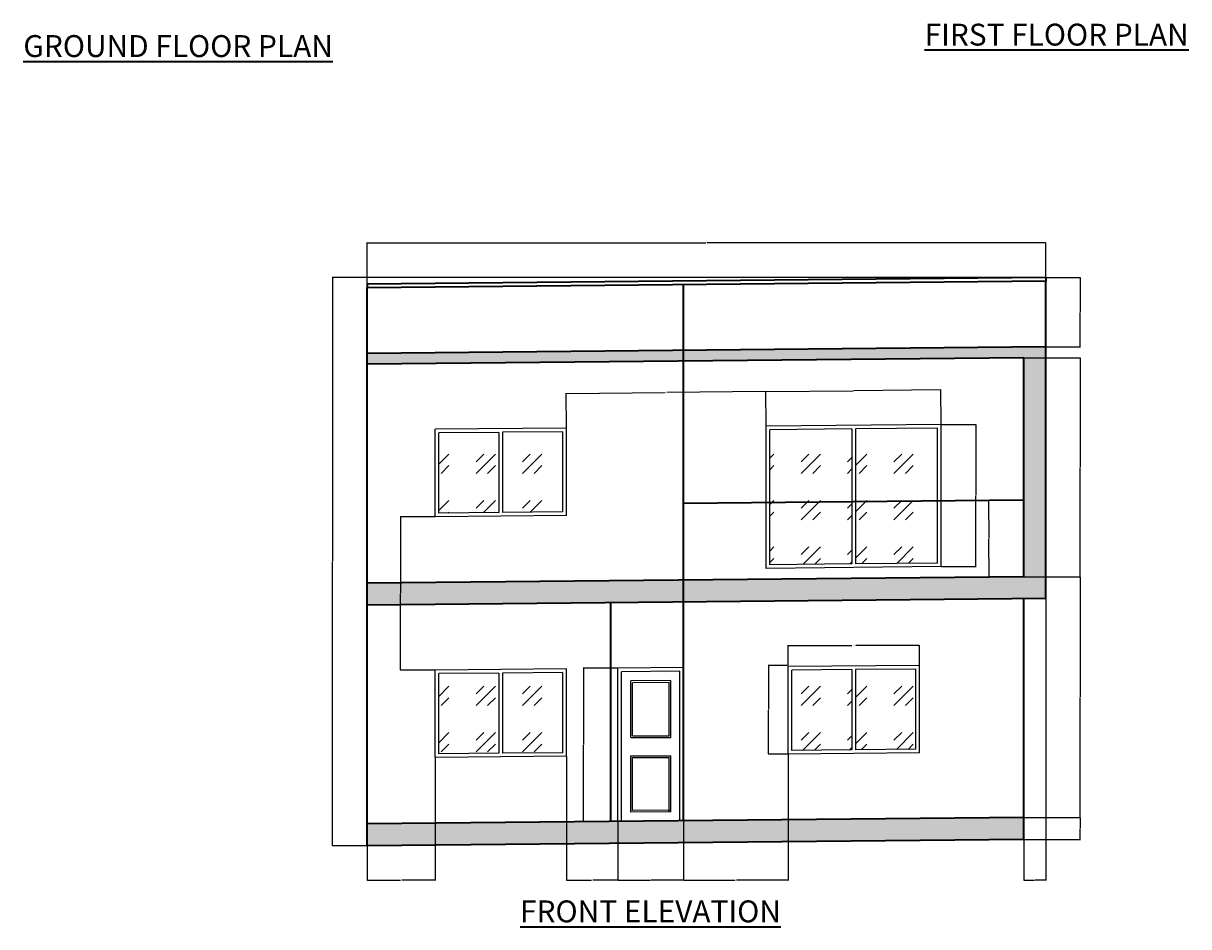
# Model space of a CAD drawing. Units: inches. Extents: x 2831 to 3729, y 3926 to 4974.
# Tile 1 of 8: x 2934 to 3573, y 3926 to 4422. Entities that reach past the tile are written whole.
import ezdxf

# ---------------------------------------------------------------- set-up
doc = ezdxf.new("R2010")
doc.units = ezdxf.units.IN
for name, color, linetype, lineweight in [('A-ANNO-DIMS', 2, 'Continuous', 18), ('A-ANNO-TEXT', 7, 'Continuous', 35), ('A-DOOR', 3, 'Continuous', 25), ('A-ELEV', 7, 'Continuous', 35), ('A-ELEV-PATT', 252, 'Continuous', 13), ('A-GLAZ', 4, 'Continuous', 25), ('A-GLAZ-PATT', 9, 'Continuous', 13)]:
    doc.layers.add(name, color=color, linetype=linetype, lineweight=lineweight)
doc.styles.get("Standard").update_dxf_attribs({"font": 'arial.ttf'})
doc.dimstyles.get("Standard").update_dxf_attribs({"dimtxt": 0.18, "dimasz": 0.18, "dimexe": 0.18, "dimexo": 0.0625, "dimgap": 0.09, "dimtad": 0, "dimtih": 1, "dimtoh": 1, "dimdec": 4, "dimzin": 0, "dimdsep": 46, "dimtxsty": 'Standard', "dimcen": 0.09, "dimadec": 0, "dimazin": 0, "dimtfac": 1, "dimtdec": 4, "dimtofl": 0, "dimtmove": 0, "dimatfit": 3, "dimfxl": 1, "dimtolj": 1, "dimtzin": 0, "dimarcsym": 0})

# ---------------------------------------------------------------- blocks, each defined once
blk = doc.blocks.new('WINDOW-72X48IN-ELEV')
for p, q in [((0, 48), (72, 48.7)), ((0, 48), (0, 0)), ((2, 46.02), (35, 46.34)), ((2, 46.02), (2, 2.02)), ((35, 2.34), (35, 46.34)), ((37, 46.36), (70, 46.68)), ((37, 2.36), (37, 46.36)), ((70, 46.68), (70, 2.68)), ((72, 48.7), (72, 0.7)), ((0, 0), (72, 0.7)), ((2, 2.02), (35, 2.34)), ((37, 2.36), (70, 2.68))]:
    blk.add_line(p, q)
blk = doc.blocks.new('*D27')
at = {"layer": 'A-ANNO-DIMS', "color": 0, "lineweight": -2, "transparency": 16777216}
for p, q in [((3353.06, 4069.58), (3353.06, 4080.49)), ((3353.24, 4080.31), (3387.94, 4080.31)), ((3424.88, 4080.31), (3390.18, 4080.31)), ((3425.06, 4069.58), (3425.06, 4080.49))]:
    blk.add_line(p, q, dxfattribs=at)
at = {"layer": 'A-ANNO-DIMS', "color": 0, "transparency": 16777216}
for points in [[(3353.24, 4080.34), (3353.24, 4080.28), (3353.06, 4080.31)], [(3424.88, 4080.34), (3424.88, 4080.28), (3425.06, 4080.31)]]:
    blk.add_solid(points, dxfattribs=at)
at = {"layer": 'Defpoints', "color": 0, "transparency": 16777216}
for p in [(3353.06, 4080.31), (3353.06, 4069.51), (3425.06, 4069.51)]:
    blk.add_point(p, dxfattribs=at)
at = {"layer": 'A-ANNO-DIMS', "color": 0, "transparency": 16777216, "insert": (3389.06, 4080.31), "char_height": 0.18, "attachment_point": 5}
blk.add_mtext('\\A1;WINDOW 72 TYP.', dxfattribs=at)
blk = doc.blocks.new('*D28')
at = {"layer": 'A-ANNO-DIMS', "color": 0, "lineweight": -2, "transparency": 16777216}
for p, q in [((3352.99, 4069.51), (3342.08, 4069.51)), ((3342.26, 4069.33), (3342.26, 4045.34)), ((3342.26, 4020.99), (3342.26, 4044.98)), ((3352.99, 4020.81), (3342.08, 4020.81))]:
    blk.add_line(p, q, dxfattribs=at)
at = {"layer": 'A-ANNO-DIMS', "color": 0, "transparency": 16777216}
for points in [[(3342.23, 4069.33), (3342.29, 4069.33), (3342.26, 4069.51)], [(3342.23, 4020.99), (3342.29, 4020.99), (3342.26, 4020.81)]]:
    blk.add_solid(points, dxfattribs=at)
at = {"layer": 'Defpoints', "color": 0, "transparency": 16777216}
for p in [(3353.06, 4069.51), (3342.26, 4020.81), (3353.06, 4020.81)]:
    blk.add_point(p, dxfattribs=at)
at = {"layer": 'A-ANNO-DIMS', "color": 0, "transparency": 16777216, "insert": (3342.26, 4045.16), "char_height": 0.18, "attachment_point": 5}
blk.add_mtext('\\A1;49 TYP.', dxfattribs=at)
blk = doc.blocks.new('*D62')
at = {"layer": 'A-ANNO-DIMS', "color": 0, "lineweight": -2, "transparency": 16777216}
for p, q in [((3122.29, 4278.64), (3122.29, 4301.33)), ((3122.47, 4301.15), (3308, 4301.15)), ((3494.11, 4301.15), (3308.58, 4301.15)), ((3494.29, 4282.26), (3494.29, 4301.33))]:
    blk.add_line(p, q, dxfattribs=at)
at = {"layer": 'A-ANNO-DIMS', "color": 0, "transparency": 16777216}
for points in [[(3122.47, 4301.18), (3122.47, 4301.12), (3122.29, 4301.15)], [(3494.11, 4301.18), (3494.11, 4301.12), (3494.29, 4301.15)]]:
    blk.add_solid(points, dxfattribs=at)
at = {"layer": 'Defpoints', "color": 0, "transparency": 16777216}
for p in [(3494.29, 4301.15), (3494.29, 4282.2), (3122.29, 4278.58)]:
    blk.add_point(p, dxfattribs=at)
at = {"layer": 'A-ANNO-DIMS', "color": 0, "transparency": 16777216, "insert": (3308.29, 4301.15), "char_height": 0.18, "attachment_point": 5}
blk.add_mtext('\\A1;372', dxfattribs=at)
blk = doc.blocks.new('*D63')
at = {"layer": 'A-ANNO-DIMS', "color": 0, "lineweight": -2, "transparency": 16777216}
for p, q in [((3494.23, 4282.2), (3103.16, 4282.2)), ((3103.34, 4282.02), (3103.34, 4126.56)), ((3103.34, 3970.75), (3103.34, 4126.2)), ((3122.24, 3970.57), (3103.16, 3970.57))]:
    blk.add_line(p, q, dxfattribs=at)
at = {"layer": 'A-ANNO-DIMS', "color": 0, "transparency": 16777216}
for points in [[(3103.31, 4282.02), (3103.37, 4282.02), (3103.34, 4282.2)], [(3103.31, 3970.75), (3103.37, 3970.75), (3103.34, 3970.57)]]:
    blk.add_solid(points, dxfattribs=at)
at = {"layer": 'Defpoints', "color": 0, "transparency": 16777216}
for p in [(3103.34, 4282.2), (3494.29, 4282.2), (3122.31, 3970.57)]:
    blk.add_point(p, dxfattribs=at)
at = {"layer": 'A-ANNO-DIMS', "color": 0, "transparency": 16777216, "insert": (3103.34, 4126.38), "char_height": 0.18, "attachment_point": 5}
blk.add_mtext('\\A1;311.6', dxfattribs=at)
blk = doc.blocks.new('*D64')
at = {"layer": 'A-ANNO-DIMS', "color": 0, "lineweight": -2, "transparency": 16777216}
for p, q in [((3482.37, 3986.07), (3513.44, 3986.07)), ((3513.26, 3985.89), (3513.26, 3980.25)), ((3482.37, 3974.07), (3513.44, 3974.07)), ((3513.26, 3974.25), (3513.26, 3979.89))]:
    blk.add_line(p, q, dxfattribs=at)
at = {"layer": 'A-ANNO-DIMS', "color": 0, "transparency": 16777216}
for points in [[(3513.23, 3985.89), (3513.29, 3985.89), (3513.26, 3986.07)], [(3513.23, 3974.25), (3513.29, 3974.25), (3513.26, 3974.07)]]:
    blk.add_solid(points, dxfattribs=at)
at = {"layer": 'Defpoints', "color": 0, "transparency": 16777216}
for p in [(3482.31, 3986.07), (3513.26, 3986.07), (3482.31, 3974.07)]:
    blk.add_point(p, dxfattribs=at)
at = {"layer": 'A-ANNO-DIMS', "color": 0, "transparency": 16777216, "insert": (3513.26, 3980.07), "char_height": 0.18, "attachment_point": 5}
blk.add_mtext('\\A1;12', dxfattribs=at)
blk = doc.blocks.new('*D65')
at = {"layer": 'A-ANNO-DIMS', "color": 0, "lineweight": -2, "transparency": 16777216}
for p, q in [((3482.37, 4118.07), (3513.44, 4118.07)), ((3513.26, 4117.89), (3513.26, 4052.25)), ((3513.26, 3986.25), (3513.26, 4051.89)), ((3482.37, 3986.07), (3513.44, 3986.07))]:
    blk.add_line(p, q, dxfattribs=at)
at = {"layer": 'A-ANNO-DIMS', "color": 0, "transparency": 16777216}
for points in [[(3513.23, 4117.89), (3513.29, 4117.89), (3513.26, 4118.07)], [(3513.23, 3986.25), (3513.29, 3986.25), (3513.26, 3986.07)]]:
    blk.add_solid(points, dxfattribs=at)
at = {"layer": 'Defpoints', "color": 0, "transparency": 16777216}
for p in [(3482.31, 4118.07), (3513.26, 4118.07), (3482.31, 3986.07)]:
    blk.add_point(p, dxfattribs=at)
at = {"layer": 'A-ANNO-DIMS', "color": 0, "transparency": 16777216, "insert": (3513.26, 4052.07), "char_height": 0.18, "attachment_point": 5}
blk.add_mtext('\\A1;132', dxfattribs=at)
blk = doc.blocks.new('*D66')
at = {"layer": 'A-ANNO-DIMS', "color": 0, "lineweight": -2, "transparency": 16777216}
for p, q in [((3482.37, 4238.08), (3513.44, 4238.08)), ((3513.26, 4237.9), (3513.26, 4178.26)), ((3513.26, 4118.25), (3513.26, 4177.89)), ((3482.37, 4118.07), (3513.44, 4118.07))]:
    blk.add_line(p, q, dxfattribs=at)
at = {"layer": 'A-ANNO-DIMS', "color": 0, "transparency": 16777216}
for points in [[(3513.23, 4237.9), (3513.29, 4237.9), (3513.26, 4238.08)], [(3513.23, 4118.25), (3513.29, 4118.25), (3513.26, 4118.07)]]:
    blk.add_solid(points, dxfattribs=at)
at = {"layer": 'Defpoints', "color": 0, "transparency": 16777216}
for p in [(3482.31, 4238.08), (3513.26, 4238.08), (3482.31, 4118.07)]:
    blk.add_point(p, dxfattribs=at)
at = {"layer": 'A-ANNO-DIMS', "color": 0, "transparency": 16777216, "insert": (3513.26, 4178.08), "char_height": 0.18, "attachment_point": 5}
blk.add_mtext('\\A1;120', dxfattribs=at)
blk = doc.blocks.new('*D67')
at = {"layer": 'A-ANNO-DIMS', "color": 0, "lineweight": -2, "transparency": 16777216}
for p, q in [((3494.35, 4282.2), (3513.44, 4282.2)), ((3513.26, 4282.02), (3513.26, 4263.38)), ((3513.26, 4244.38), (3513.26, 4263.01)), ((3494.37, 4244.2), (3513.44, 4244.2))]:
    blk.add_line(p, q, dxfattribs=at)
at = {"layer": 'A-ANNO-DIMS', "color": 0, "transparency": 16777216}
for points in [[(3513.23, 4282.02), (3513.29, 4282.02), (3513.26, 4282.2)], [(3513.23, 4244.38), (3513.29, 4244.38), (3513.26, 4244.2)]]:
    blk.add_solid(points, dxfattribs=at)
at = {"layer": 'Defpoints', "color": 0, "transparency": 16777216}
for p in [(3494.29, 4282.2), (3513.26, 4282.2), (3494.31, 4244.2)]:
    blk.add_point(p, dxfattribs=at)
at = {"layer": 'A-ANNO-DIMS', "color": 0, "transparency": 16777216, "insert": (3513.26, 4263.2), "char_height": 0.18, "attachment_point": 5}
blk.add_mtext('\\A1;38', dxfattribs=at)
blk = doc.blocks.new('*D68')
at = {"layer": 'A-ANNO-DIMS', "color": 0, "lineweight": -2, "transparency": 16777216}
for p, q in [((3159.56, 4018.87), (3159.56, 3951.44)), ((3122.31, 3970.5), (3122.31, 3951.44)), ((3122.49, 3951.62), (3140.54, 3951.62)), ((3159.38, 3951.62), (3141.33, 3951.62))]:
    blk.add_line(p, q, dxfattribs=at)
at = {"layer": 'A-ANNO-DIMS', "color": 0, "transparency": 16777216}
for points in [[(3122.49, 3951.65), (3122.49, 3951.59), (3122.31, 3951.62)], [(3159.38, 3951.65), (3159.38, 3951.59), (3159.56, 3951.62)]]:
    blk.add_solid(points, dxfattribs=at)
at = {"layer": 'Defpoints', "color": 0, "transparency": 16777216}
for p in [(3159.56, 4018.93), (3122.31, 3970.57), (3159.56, 3951.62)]:
    blk.add_point(p, dxfattribs=at)
at = {"layer": 'A-ANNO-DIMS', "color": 0, "transparency": 16777216, "insert": (3140.93, 3951.62), "char_height": 0.18, "attachment_point": 5}
blk.add_mtext('\\A1;37.25', dxfattribs=at)
blk = doc.blocks.new('*D69')
at = {"layer": 'A-ANNO-DIMS', "color": 0, "lineweight": -2, "transparency": 16777216}
for p, q in [((3231.56, 4019.57), (3231.56, 3951.44)), ((3259.81, 3983.84), (3259.81, 3951.44)), ((3231.74, 3951.62), (3245.29, 3951.62)), ((3259.63, 3951.62), (3246.08, 3951.62))]:
    blk.add_line(p, q, dxfattribs=at)
at = {"layer": 'A-ANNO-DIMS', "color": 0, "transparency": 16777216}
for points in [[(3231.74, 3951.65), (3231.74, 3951.59), (3231.56, 3951.62)], [(3259.63, 3951.65), (3259.63, 3951.59), (3259.81, 3951.62)]]:
    blk.add_solid(points, dxfattribs=at)
at = {"layer": 'Defpoints', "color": 0, "transparency": 16777216}
for p in [(3231.56, 4019.63), (3259.81, 3983.9), (3259.81, 3951.62)]:
    blk.add_point(p, dxfattribs=at)
at = {"layer": 'A-ANNO-DIMS', "color": 0, "transparency": 16777216, "insert": (3245.68, 3951.62), "char_height": 0.18, "attachment_point": 5}
blk.add_mtext('\\A1;28.25', dxfattribs=at)
blk = doc.blocks.new('*D70')
at = {"layer": 'A-ANNO-DIMS', "color": 0, "lineweight": -2, "transparency": 16777216}
for p, q in [((3259.81, 3983.84), (3259.81, 3951.44)), ((3295.81, 3984.19), (3295.81, 3951.44)), ((3259.99, 3951.62), (3277.59, 3951.62)), ((3295.63, 3951.62), (3278.03, 3951.62))]:
    blk.add_line(p, q, dxfattribs=at)
at = {"layer": 'A-ANNO-DIMS', "color": 0, "transparency": 16777216}
for points in [[(3259.99, 3951.65), (3259.99, 3951.59), (3259.81, 3951.62)], [(3295.63, 3951.65), (3295.63, 3951.59), (3295.81, 3951.62)]]:
    blk.add_solid(points, dxfattribs=at)
at = {"layer": 'Defpoints', "color": 0, "transparency": 16777216}
for p in [(3259.81, 3983.9), (3295.81, 3984.25), (3295.81, 3951.62)]:
    blk.add_point(p, dxfattribs=at)
at = {"layer": 'A-ANNO-DIMS', "color": 0, "transparency": 16777216, "insert": (3277.81, 3951.62), "char_height": 0.18, "attachment_point": 5}
blk.add_mtext('\\A1;36', dxfattribs=at)
blk = doc.blocks.new('*D71')
at = {"layer": 'A-ANNO-DIMS', "color": 0, "lineweight": -2, "transparency": 16777216}
for p, q in [((3353.06, 4020.75), (3353.06, 3951.44)), ((3295.81, 3984.19), (3295.81, 3951.44)), ((3295.99, 3951.62), (3324.04, 3951.62)), ((3352.88, 3951.62), (3324.83, 3951.62))]:
    blk.add_line(p, q, dxfattribs=at)
at = {"layer": 'A-ANNO-DIMS', "color": 0, "transparency": 16777216}
for points in [[(3295.99, 3951.65), (3295.99, 3951.59), (3295.81, 3951.62)], [(3352.88, 3951.65), (3352.88, 3951.59), (3353.06, 3951.62)]]:
    blk.add_solid(points, dxfattribs=at)
at = {"layer": 'Defpoints', "color": 0, "transparency": 16777216}
for p in [(3353.06, 4020.81), (3295.81, 3984.25), (3353.06, 3951.62)]:
    blk.add_point(p, dxfattribs=at)
at = {"layer": 'A-ANNO-DIMS', "color": 0, "transparency": 16777216, "insert": (3324.43, 3951.62), "char_height": 0.18, "attachment_point": 5}
blk.add_mtext('\\A1;57.25', dxfattribs=at)
blk = doc.blocks.new('*D72')
at = {"layer": 'A-ANNO-DIMS', "color": 0, "lineweight": -2, "transparency": 16777216}
for p, q in [((3341.06, 4200.77), (3340.87, 4219.83)), ((3341.05, 4219.65), (3388.65, 4220.12)), ((3436.69, 4220.58), (3389.09, 4220.12)), ((3437.06, 4201.7), (3436.87, 4220.77))]:
    blk.add_line(p, q, dxfattribs=at)
at = {"layer": 'A-ANNO-DIMS', "color": 0, "transparency": 16777216}
for points in [[(3341.05, 4219.68), (3341.05, 4219.62), (3340.87, 4219.65)], [(3436.69, 4220.61), (3436.69, 4220.55), (3436.87, 4220.59)]]:
    blk.add_solid(points, dxfattribs=at)
at = {"layer": 'Defpoints', "color": 0, "transparency": 16777216}
for p in [(3436.87, 4220.59), (3341.06, 4200.7), (3437.06, 4201.64)]:
    blk.add_point(p, dxfattribs=at)
at = {"layer": 'A-ANNO-DIMS', "color": 0, "transparency": 16777216, "insert": (3388.87, 4220.12), "char_height": 0.18, "attachment_point": 5}
blk.add_mtext('\\A1;96', dxfattribs=at)
blk = doc.blocks.new('*D73')
at = {"layer": 'A-ANNO-DIMS', "color": 0, "lineweight": -2, "transparency": 16777216}
for p, q in [((3231.56, 4199.7), (3231.37, 4218.77)), ((3231.55, 4218.59), (3285.74, 4219.12)), ((3340.69, 4219.65), (3286.51, 4219.12)), ((3341.06, 4200.77), (3340.87, 4219.83))]:
    blk.add_line(p, q, dxfattribs=at)
at = {"layer": 'A-ANNO-DIMS', "color": 0, "transparency": 16777216}
for points in [[(3231.55, 4218.62), (3231.55, 4218.56), (3231.37, 4218.59)], [(3340.69, 4219.68), (3340.69, 4219.62), (3340.87, 4219.65)]]:
    blk.add_solid(points, dxfattribs=at)
at = {"layer": 'Defpoints', "color": 0, "transparency": 16777216}
for p in [(3340.87, 4219.65), (3231.56, 4199.64), (3341.06, 4200.7)]:
    blk.add_point(p, dxfattribs=at)
at = {"layer": 'A-ANNO-DIMS', "color": 0, "transparency": 16777216, "insert": (3286.12, 4219.12), "char_height": 0.18, "attachment_point": 5}
blk.add_mtext('\\A1;109.5', dxfattribs=at)
blk = doc.blocks.new('*D74')
at = {"layer": 'A-ANNO-DIMS', "color": 0, "lineweight": -2, "transparency": 16777216}
for p, q in [((3437.12, 4201.64), (3456.19, 4201.64)), ((3456.01, 4201.46), (3456.01, 4162.82)), ((3456.01, 4123.81), (3456.01, 4162.45)), ((3437.12, 4123.63), (3456.19, 4123.63))]:
    blk.add_line(p, q, dxfattribs=at)
at = {"layer": 'A-ANNO-DIMS', "color": 0, "transparency": 16777216}
for points in [[(3455.98, 4201.46), (3456.04, 4201.46), (3456.01, 4201.64)], [(3455.98, 4123.81), (3456.04, 4123.81), (3456.01, 4123.63)]]:
    blk.add_solid(points, dxfattribs=at)
at = {"layer": 'Defpoints', "color": 0, "transparency": 16777216}
for p in [(3437.06, 4201.64), (3437.06, 4123.63), (3456.01, 4123.63)]:
    blk.add_point(p, dxfattribs=at)
at = {"layer": 'A-ANNO-DIMS', "color": 0, "transparency": 16777216, "insert": (3456.01, 4162.63), "char_height": 0.18, "attachment_point": 5}
blk.add_mtext('\\A1;78', dxfattribs=at)
blk = doc.blocks.new('*D75')
at = {"layer": 'A-ANNO-DIMS', "color": 0, "lineweight": -2, "transparency": 16777216}
for p, q in [((3259.74, 4067.91), (3240.68, 4067.91)), ((3240.86, 4067.73), (3240.86, 4026.09)), ((3240.86, 3984.08), (3240.86, 4025.72)), ((3259.74, 3983.9), (3240.68, 3983.9))]:
    blk.add_line(p, q, dxfattribs=at)
at = {"layer": 'A-ANNO-DIMS', "color": 0, "transparency": 16777216}
for points in [[(3240.83, 4067.73), (3240.89, 4067.73), (3240.86, 4067.91)], [(3240.83, 3984.08), (3240.89, 3984.08), (3240.86, 3983.9)]]:
    blk.add_solid(points, dxfattribs=at)
at = {"layer": 'Defpoints', "color": 0, "transparency": 16777216}
for p in [(3240.86, 4067.91), (3259.81, 4067.91), (3259.81, 3983.9)]:
    blk.add_point(p, dxfattribs=at)
at = {"layer": 'A-ANNO-DIMS', "color": 0, "transparency": 16777216, "insert": (3240.86, 4025.91), "char_height": 0.18, "attachment_point": 5}
blk.add_mtext('\\A1;84', dxfattribs=at)
blk = doc.blocks.new('*D76')
at = {"layer": 'A-ANNO-DIMS', "color": 0, "lineweight": -2, "transparency": 16777216}
for p, q in [((3159.49, 4150.94), (3140.43, 4150.94)), ((3140.61, 4150.76), (3140.61, 4109.12)), ((3140.61, 4067.11), (3140.61, 4108.75)), ((3159.49, 4066.93), (3140.43, 4066.93))]:
    blk.add_line(p, q, dxfattribs=at)
at = {"layer": 'A-ANNO-DIMS', "color": 0, "transparency": 16777216}
for points in [[(3140.58, 4150.76), (3140.64, 4150.76), (3140.61, 4150.94)], [(3140.58, 4067.11), (3140.64, 4067.11), (3140.61, 4066.93)]]:
    blk.add_solid(points, dxfattribs=at)
at = {"layer": 'Defpoints', "color": 0, "transparency": 16777216}
for p in [(3140.61, 4150.94), (3159.56, 4150.94), (3159.56, 4066.93)]:
    blk.add_point(p, dxfattribs=at)
at = {"layer": 'A-ANNO-DIMS', "color": 0, "transparency": 16777216, "insert": (3140.61, 4108.94), "char_height": 0.18, "attachment_point": 5}
blk.add_mtext('\\A1;84', dxfattribs=at)
blk = doc.blocks.new('*D77')
at = {"layer": 'A-ANNO-DIMS', "color": 0, "lineweight": -2, "transparency": 16777216}
for p, q in [((3481.84, 4160.07), (3462.77, 4159.88)), ((3462.95, 4159.71), (3463.15, 4139.07)), ((3463.36, 4118.07), (3463.16, 4138.71)), ((3482.24, 4118.07), (3463.18, 4117.89))]:
    blk.add_line(p, q, dxfattribs=at)
at = {"layer": 'A-ANNO-DIMS', "color": 0, "transparency": 16777216}
for points in [[(3462.98, 4159.71), (3462.92, 4159.71), (3462.95, 4159.89)], [(3463.39, 4118.07), (3463.33, 4118.07), (3463.36, 4117.89)]]:
    blk.add_solid(points, dxfattribs=at)
at = {"layer": 'Defpoints', "color": 0, "transparency": 16777216}
for p in [(3462.95, 4159.89), (3481.9, 4160.07), (3482.31, 4118.07)]:
    blk.add_point(p, dxfattribs=at)
at = {"layer": 'A-ANNO-DIMS', "color": 0, "transparency": 16777216, "insert": (3463.15, 4138.89), "char_height": 0.18, "attachment_point": 5}
blk.add_mtext('\\A1;42', dxfattribs=at)
blk = doc.blocks.new('*D78')
at = {"layer": 'A-ANNO-DIMS', "color": 0, "lineweight": -2, "transparency": 16777216}
for p, q in [((3494.31, 4106.13), (3494.31, 3951.44)), ((3482.31, 3974), (3482.31, 3951.44)), ((3482.49, 3951.62), (3488.1, 3951.62)), ((3494.13, 3951.62), (3488.52, 3951.62))]:
    blk.add_line(p, q, dxfattribs=at)
at = {"layer": 'A-ANNO-DIMS', "color": 0, "transparency": 16777216}
for points in [[(3482.49, 3951.65), (3482.49, 3951.59), (3482.31, 3951.62)], [(3494.13, 3951.65), (3494.13, 3951.59), (3494.31, 3951.62)]]:
    blk.add_solid(points, dxfattribs=at)
at = {"layer": 'Defpoints', "color": 0, "transparency": 16777216}
for p in [(3494.31, 4106.19), (3482.31, 3974.07), (3494.31, 3951.62)]:
    blk.add_point(p, dxfattribs=at)
at = {"layer": 'A-ANNO-DIMS', "color": 0, "transparency": 16777216, "insert": (3488.31, 3951.62), "char_height": 0.18, "attachment_point": 5}
blk.add_mtext('\\A1;12', dxfattribs=at)

msp = doc.modelspace()

# ---------------------------------------------------------------- hatches: boundary and pattern name
at = {"layer": 'A-ELEV-PATT'}
h = msp.add_hatch(color=256, dxfattribs=at)
h.dxf.hatch_style = 1
h.paths.add_polyline_path([(3295.8071, 4242.2662), (3122.3071, 4240.5802), (3122.3071, 4234.5799), (3295.8071, 4236.2659)])
h = msp.add_hatch(color=256, dxfattribs=at)
h.dxf.hatch_style = 1
h.paths.add_polyline_path([(3494.3071, 4244.1951), (3295.8071, 4242.2662), (3295.8071, 4236.2659), (3482.3071, 4238.0782), (3482.3071, 4118.0726), (3295.8071, 4116.2602), (3295.8071, 4104.2597), (3494.3071, 4106.1886)])
h = msp.add_hatch(color=256, dxfattribs=at)
h.dxf.hatch_style = 1
h.paths.add_polyline_path([(3295.8071, 4116.2602), (3122.3071, 4114.5743), (3122.3071, 4102.5737), (3295.8071, 4104.2597)])
h = msp.add_hatch(color=256, dxfattribs=at)
h.dxf.hatch_style = 1
h.paths.add_polyline_path([(3482.3071, 3986.0663), (3122.3071, 3982.568), (3122.3071, 3970.5675), (3482.3071, 3974.0658)])
at = {"layer": 'A-GLAZ-PATT'}
h = msp.add_hatch(dxfattribs=at)
h.set_pattern_fill('GOST_GLASS', color=256, scale=3)
h.paths.add_polyline_path([(3194.5571, 4197.2802), (3161.5571, 4196.9595), (3161.5571, 4152.9575), (3194.5571, 4153.2781)])
h.paths.add_polyline_path([(3229.5571, 4197.6203), (3196.5571, 4197.2996), (3196.5571, 4153.2976), (3229.5571, 4153.6183)])
h.paths.add_polyline_path([(3194.5571, 4065.274), (3161.5571, 4064.9533), (3161.5571, 4020.9512), (3194.5571, 4021.2719)])
h.paths.add_polyline_path([(3229.5571, 4065.6141), (3196.5571, 4065.2934), (3196.5571, 4021.2913), (3229.5571, 4021.612)])
h.paths.add_polyline_path([(3388.0571, 4067.1543), (3355.0571, 4066.8336), (3355.0571, 4022.8316), (3388.0571, 4023.1522)])
h.paths.add_polyline_path([(3423.0571, 4067.4944), (3390.0571, 4067.1738), (3390.0571, 4023.1717), (3423.0571, 4023.4924)])
h.paths.add_polyline_path([(3388.0571, 4159.1587), (3343.0571, 4158.7214), (3343.0571, 4124.7198), (3388.0571, 4125.1571)])
h.paths.add_polyline_path([(3388.0571, 4199.1606), (3343.0571, 4198.7233), (3343.0571, 4158.7214), (3388.0571, 4159.1587)])
h.paths.add_polyline_path([(3435.0571, 4199.6173), (3390.0571, 4199.18), (3390.0571, 4159.1781), (3435.0571, 4159.6154)])
h.paths.add_polyline_path([(3435.0571, 4159.6154), (3390.0571, 4159.1781), (3390.0571, 4125.1765), (3435.0571, 4125.6138)])

# ---------------------------------------------------------------- linework, layer by layer
at = {"layer": 'A-DOOR'}
for p, q in [((3437.0571, 4201.6368), (3341.0571, 4200.7039)), ((3341.0571, 4122.7002), (3341.0571, 4200.7039)), ((3388.0571, 4199.1606), (3343.0571, 4198.7233)), ((3343.0571, 4124.7198), (3343.0571, 4198.7233)), ((3388.0571, 4199.1606), (3388.0571, 4125.1571)), ((3435.0571, 4199.6173), (3390.0571, 4199.18)), ((3390.0571, 4199.18), (3390.0571, 4125.1765)), ((3435.0571, 4125.6138), (3435.0571, 4199.6173)), ((3437.0571, 4123.6331), (3437.0571, 4201.6368)), ((3437.0571, 4123.6331), (3341.0571, 4122.7002)), ((3388.0571, 4125.1571), (3343.0571, 4124.7198)), ((3435.0571, 4125.6138), (3390.0571, 4125.1765)), ((3295.8071, 4068.258), (3259.8071, 4067.9081)), ((3259.8071, 3983.9042), (3259.8071, 4067.9081)), ((3293.8071, 4066.2384), (3261.8071, 4065.9275)), ((3261.8071, 3983.9042), (3261.8071, 4065.9275)), ((3293.8071, 3984.254), (3293.8071, 4066.2384)), ((3288.8071, 4061.1896), (3266.8071, 4060.9758)), ((3266.8071, 4029.9158), (3266.8071, 4060.9758)), ((3287.8071, 4060.1799), (3267.8071, 4059.9855)), ((3267.8071, 4030.9158), (3267.8071, 4059.9855)), ((3287.8071, 4030.9158), (3287.8071, 4060.1799)), ((3288.8071, 4029.9158), (3288.8071, 4061.1896)), ((3266.8071, 4029.9158), (3288.8071, 4029.9158)), ((3267.8071, 4030.9158), (3287.8071, 4030.9158)), ((3266.8071, 4019.9158), (3288.8071, 4019.9158)), ((3266.8071, 3988.9724), (3266.8071, 4019.9158)), ((3267.8071, 4018.9158), (3287.8071, 4018.9158)), ((3267.8071, 3989.9822), (3267.8071, 4018.9158)), ((3287.8071, 3989.1862), (3287.8071, 4018.9158)), ((3288.8071, 3989.1862), (3288.8071, 4019.9158)), ((3288.8071, 3989.1862), (3266.8071, 3988.9724)), ((3288.7974, 3990.1862), (3267.8071, 3989.9822))]:
    msp.add_line(p, q, dxfattribs=at)
at = {"layer": 'A-ELEV'}
for p, q in [((3494.2877, 4282.1967), (3122.2877, 4278.5818)), ((3494.2877, 4282.1967), (3494.3071, 4280.1968)), ((3122.2877, 4278.5818), (3122.3071, 4276.5819)), ((3494.3071, 4280.1968), (3122.3071, 4276.5819)), ((3122.3071, 3970.5675), (3122.3071, 4276.5819)), ((3295.8071, 3984.254), (3295.8071, 4278.2679)), ((3494.3071, 4106.1886), (3494.3071, 4280.1968)), ((3494.3071, 4244.1951), (3122.3071, 4240.5802)), ((3482.3071, 4238.0782), (3122.3071, 4234.5799)), ((3482.3071, 4118.0726), (3482.3071, 4238.0782)), ((3481.899, 4160.0706), (3295.8071, 4158.2622)), ((3482.3071, 4118.0726), (3122.3071, 4114.5743)), ((3494.3071, 4106.1886), (3122.3071, 4102.5737)), ((3255.8071, 3983.9042), (3255.8071, 4103.871)), ((3482.3071, 3974.0658), (3482.3071, 4106.072)), ((3482.3071, 3986.0663), (3122.3071, 3982.568)), ((3482.3071, 3974.0658), (3122.3071, 3970.5675))]:
    msp.add_line(p, q, dxfattribs=at)
at = {"layer": 'A-GLAZ'}
for p, q in [((3194.5571, 4199.29), (3194.5571, 4199.2803)), ((3196.5571, 4151.2975), (3196.5571, 4151.2878))]:
    msp.add_line(p, q, dxfattribs=at)

# ---------------------------------------------------------------- block references
at = {"layer": 'A-GLAZ', "rotation": 180}
for p in [(3231.5571, 4199.6399), (3231.5571, 4067.6336), (3425.0571, 4069.514)]:
    msp.add_blockref('WINDOW-72X48IN-ELEV', p, dxfattribs=at)

# ---------------------------------------------------------------- texts
at = {"layer": 'A-ANNO-TEXT', "char_height": 12, "attachment_point": 1}
for s, insert in [('{\\LFIRST FLOOR PLAN}', (3427.8943, 4421.3727)), ('{\\LGROUND FLOOR PLAN}', (2933.7984, 4415.1046)), ('{\\LFRONT ELEVATION}', (3206.118, 3940.5944))]:
    msp.add_mtext_dynamic_manual_height_columns(s, width=274.330481, gutter_width=12.5, heights=[0], dxfattribs=dict(at, insert=insert))

# ---------------------------------------------------------------- dimensions: what is measured, and where the dimension line sits
at = {"layer": 'A-ANNO-DIMS'}
for base, p1, p2, override, picture, middle in [((3494.2877, 4301.1467), (3122.2877, 4278.5818), (3494.2877, 4282.1967), {"dimdec": 0, "dimlfac": 1, "dimrnd": 0, "dimzin": 0, "dimdsep": 46, "dimlunit": 2}, '*D62', (3308.2877, 4301.1467)), ((3494.3071, 3951.6175), (3482.3071, 3974.0658), (3494.3071, 4106.1886), {"dimdec": 0, "dimlfac": 1, "dimrnd": 0, "dimzin": 0, "dimdsep": 46, "dimlunit": 2}, '*D78', (3488.3071, 3951.6175)), ((3159.5571, 3951.6175), (3122.3071, 3970.5675), (3159.5571, 4018.9317), {"dimdec": 2, "dimlfac": 1, "dimrnd": 0, "dimzin": 0, "dimdsep": 46, "dimlunit": 2}, '*D68', (3140.9321, 3951.6175)), ((3259.8071, 3951.6175), (3231.5571, 4019.6314), (3259.8071, 3983.9042), {"dimdec": 2, "dimlfac": 1, "dimrnd": 0, "dimzin": 0, "dimdsep": 46, "dimlunit": 2}, '*D69', (3245.6821, 3951.6175)), ((3353.0571, 3951.6175), (3295.8071, 3984.254), (3353.0571, 4020.812), {"dimdec": 2, "dimlfac": 1, "dimrnd": 0, "dimzin": 0, "dimdsep": 46, "dimlunit": 2}, '*D71', (3324.4321, 3951.6175)), ((3295.8071, 3951.6175), (3259.8071, 3983.9042), (3295.8071, 3984.254), {"dimdec": 0, "dimlfac": 1, "dimrnd": 0, "dimzin": 0, "dimdsep": 46, "dimlunit": 2}, '*D70', (3277.8071, 3951.6175))]:
    dim = msp.add_linear_dim(base=base, p1=p1, p2=p2, dimstyle='Standard', override=override, dxfattribs=at)
    dim.commit()
    dim.dimension.update_dxf_attribs({"geometry": picture, "text_midpoint": middle})
for base, p1, p2, angle, override, picture, middle in [((3103.3377, 4282.1967), (3122.3071, 3970.5675), (3494.2877, 4282.1967), 90, {"dimdec": 1, "dimlfac": 1, "dimrnd": 0, "dimzin": 0, "dimdsep": 46, "dimlunit": 2}, '*D63', (3103.3377, 4126.3821)), ((3513.2571, 4282.1967), (3494.3071, 4244.1951), (3494.2877, 4282.1967), 90, {"dimdec": 0, "dimlfac": 1, "dimrnd": 0, "dimzin": 0, "dimdsep": 46, "dimlunit": 2}, '*D67', (3513.2571, 4263.1959)), ((3513.2571, 4238.0782), (3482.3071, 4118.0726), (3482.3071, 4238.0782), 90, {"dimdec": 0, "dimlfac": 1, "dimrnd": 0, "dimzin": 0, "dimdsep": 46, "dimlunit": 2}, '*D66', (3513.2571, 4178.0754)), ((3340.873, 4219.653), (3231.5571, 4199.6399), (3341.0571, 4200.7039), 0.5567557, {"dimdec": 1, "dimlfac": 1, "dimrnd": 0, "dimzin": 0, "dimdsep": 46, "dimlunit": 2}, '*D73', (3286.123, 4219.121)), ((3436.873, 4220.5859), (3341.0571, 4200.7039), (3437.0571, 4201.6368), 0.5567557, {"dimdec": 0, "dimlfac": 1, "dimrnd": 0, "dimzin": 0, "dimdsep": 46, "dimlunit": 2}, '*D72', (3388.873, 4220.1195)), ((3456.0071, 4123.6331), (3437.0571, 4201.6368), (3437.0571, 4123.6331), 270, {"dimdec": 0, "dimlfac": 1, "dimrnd": 0, "dimzin": 0, "dimdsep": 46, "dimlunit": 2}, '*D74', (3456.0071, 4162.635)), ((3462.9499, 4159.8864), (3482.3071, 4118.0726), (3481.899, 4160.0706), 90.5567557, {"dimdec": 0, "dimlfac": 1, "dimrnd": 0, "dimzin": 0, "dimdsep": 46, "dimlunit": 2}, '*D77', (3463.154, 4138.8874)), ((3140.6071, 4150.9379), (3159.5571, 4066.934), (3159.5571, 4150.9379), 90, {"dimdec": 0, "dimlfac": 1, "dimrnd": 0, "dimzin": 0, "dimdsep": 46, "dimlunit": 2}, '*D76', (3140.6071, 4108.9359)), ((3513.2571, 4118.0726), (3482.3071, 3986.0663), (3482.3071, 4118.0726), 90, {"dimdec": 0, "dimlfac": 1, "dimrnd": 0, "dimzin": 0, "dimdsep": 46, "dimlunit": 2}, '*D65', (3513.2571, 4052.0694)), ((3240.8571, 4067.9081), (3259.8071, 3983.9042), (3259.8071, 4067.9081), 90, {"dimdec": 0, "dimlfac": 1, "dimrnd": 0, "dimzin": 0, "dimdsep": 46, "dimlunit": 2}, '*D75', (3240.8571, 4025.9062)), ((3513.2571, 3986.0663), (3482.3071, 3974.0658), (3482.3071, 3986.0663), 90, {"dimdec": 0, "dimlfac": 1, "dimrnd": 0, "dimzin": 0, "dimdsep": 46, "dimlunit": 2}, '*D64', (3513.2571, 3980.066))]:
    dim = msp.add_linear_dim(base=base, p1=p1, p2=p2, angle=angle, dimstyle='Standard', override=override, dxfattribs=at)
    dim.commit()
    dim.dimension.update_dxf_attribs({"geometry": picture, "text_midpoint": middle})
for base, p1, p2, angle, text, picture, middle in [((3353.0571, 4080.314), (3425.0571, 4069.514), (3353.0571, 4069.514), 180, 'WINDOW <> TYP.', '*D27', (3389.0571, 4080.314)), ((3342.2571, 4020.812), (3353.0571, 4069.514), (3353.0571, 4020.812), 270, '<> TYP.', '*D28', (3342.2571, 4045.163))]:
    dim = msp.add_linear_dim(base=base, p1=p1, p2=p2, angle=angle, text=text, dimstyle='Standard', override={"dimdec": 0, "dimlfac": 1, "dimrnd": 0, "dimzin": 0, "dimdsep": 46, "dimlunit": 2}, dxfattribs=at)
    dim.commit()
    dim.dimension.update_dxf_attribs({"geometry": picture, "text_midpoint": middle})

doc.saveas('drawing.dxf')
